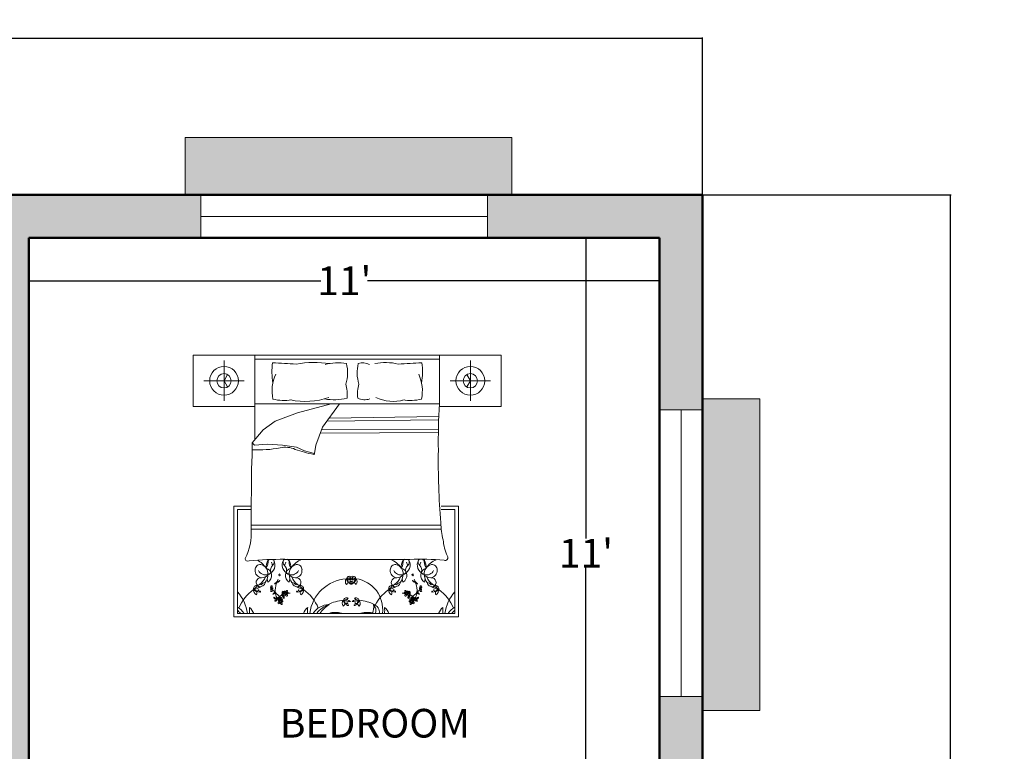
# Model space of a CAD drawing. Units: inches. Extents: x -28 to 544, y -640 to 52.
# Tile 11 of 11: x 338 to 544, y -109 to 44. Entities that reach past the tile are written whole.
import ezdxf

# ---------------------------------------------------------------- set-up
doc = ezdxf.new("R2010")
doc.units = ezdxf.units.IN
doc.header["$MEASUREMENT"] = 0
for name, color, linetype, lineweight in [('A-ANNO-DIMS', 2, 'Continuous', 18), ('A-AREA-IDEN', 7, 'Continuous', 25), ('A-FURN', 8, 'Continuous', 18), ('A-GLAZ', 4, 'Continuous', 20), ('A-ROOF', 8, 'Continuous', 18), ('A-ROOF-PATT', 252, 'Continuous', 13), ('A-WALL', 7, 'Continuous', 50), ('A-WALL-PATT', 5, 'Continuous', 13)]:
    doc.layers.add(name, color=color, linetype=linetype, lineweight=lineweight)
doc.styles.get("Standard").update_dxf_attribs({"font": 'arial.ttf'})
doc.dimstyles.get("Standard").update_dxf_attribs({"dimtxt": 0.18, "dimasz": 0.18, "dimexe": 0.18, "dimexo": 0.0625, "dimgap": 0.09, "dimtad": 0, "dimtih": 1, "dimtoh": 1, "dimdec": 0, "dimzin": 0, "dimdsep": 46, "dimlunit": 3, "dimtxsty": 'Standard', "dimcen": 0.09, "dimadec": 0, "dimazin": 0, "dimtfac": 1, "dimtdec": 0, "dimtofl": 0, "dimtmove": 0, "dimatfit": 3, "dimfxl": 1, "dimtolj": 1, "dimtzin": 0, "dimarcsym": 0})

# ---------------------------------------------------------------- blocks, each defined once
blk = doc.blocks.new('*D7')
at = {"layer": 'A-ANNO-DIMS', "color": 0, "lineweight": -2, "transparency": 16777216}
for p, q in [((456.03, -1.42), (456.03, -64.14)), ((456.09, -1.24), (456.21, -1.24)), ((456.03, -133.06), (456.03, -70.34)), ((456.09, -133.24), (456.21, -133.24))]:
    blk.add_line(p, q, dxfattribs=at)
at = {"layer": 'A-ANNO-DIMS', "color": 0, "transparency": 16777216}
for points in [[(456, -1.42), (456.06, -1.42), (456.03, -1.24)], [(456, -133.06), (456.06, -133.06), (456.03, -133.24)]]:
    blk.add_solid(points, dxfattribs=at)
at = {"layer": 'Defpoints', "color": 0, "transparency": 16777216}
for p in [(456.03, -1.24), (456.03, -133.24), (456.03, -133.24)]:
    blk.add_point(p, dxfattribs=at)
at = {"layer": 'A-ANNO-DIMS', "color": 0, "transparency": 16777216, "insert": (456.03, -67.24), "char_height": 6, "attachment_point": 5}
blk.add_mtext("\\A1;11'", dxfattribs=at)
blk = doc.blocks.new('*D8')
at = {"layer": 'A-ANNO-DIMS', "color": 0, "lineweight": -2, "transparency": 16777216}
for p, q in [((339.44, -16.04), (339.44, -10.04)), ((339.62, -10.22), (400.55, -10.22)), ((471.26, -10.22), (410.34, -10.22)), ((471.44, -16.04), (471.44, -10.04))]:
    blk.add_line(p, q, dxfattribs=at)
at = {"layer": 'A-ANNO-DIMS', "color": 0, "transparency": 16777216}
for points in [[(339.62, -10.19), (339.62, -10.25), (339.44, -10.22)], [(471.26, -10.19), (471.26, -10.25), (471.44, -10.22)]]:
    blk.add_solid(points, dxfattribs=at)
at = {"layer": 'Defpoints', "color": 0, "transparency": 16777216}
for p in [(471.44, -10.22), (339.44, -16.1), (471.44, -16.1)]:
    blk.add_point(p, dxfattribs=at)
at = {"layer": 'A-ANNO-DIMS', "color": 0, "transparency": 16777216, "insert": (405.44, -10.22), "char_height": 6, "attachment_point": 5}
blk.add_mtext("\\A1;11'", dxfattribs=at)
blk = doc.blocks.new('*D27')
at = {"layer": 'A-ANNO-DIMS', "color": 0, "lineweight": -2, "transparency": 16777216}
for p, q in [((16.94, 7.82), (16.94, 40.69)), ((17.12, 40.51), (238.3, 40.51)), ((480.26, 40.51), (259.09, 40.51)), ((480.44, 7.82), (480.44, 40.69))]:
    blk.add_line(p, q, dxfattribs=at)
at = {"layer": 'A-ANNO-DIMS', "color": 0, "transparency": 16777216}
for points in [[(17.12, 40.54), (17.12, 40.48), (16.94, 40.51)], [(480.26, 40.54), (480.26, 40.48), (480.44, 40.51)]]:
    blk.add_solid(points, dxfattribs=at)
at = {"layer": 'Defpoints', "color": 0, "transparency": 16777216}
for p in [(480.44, 40.51), (16.94, 7.76), (480.44, 7.76)]:
    blk.add_point(p, dxfattribs=at)
at = {"layer": 'A-ANNO-DIMS', "color": 0, "transparency": 16777216, "insert": (248.69, 40.51), "char_height": 6, "attachment_point": 5}
blk.add_mtext('\\A1;38\'-8"', dxfattribs=at)
blk = doc.blocks.new('*D28')
at = {"layer": 'A-ANNO-DIMS', "color": 0, "lineweight": -2, "transparency": 16777216}
for p, q in [((480.51, 7.76), (532.47, 7.76)), ((532.29, 7.58), (532.29, -286.84)), ((532.29, -587.56), (532.29, -293.14)), ((480.51, -587.74), (532.47, -587.74))]:
    blk.add_line(p, q, dxfattribs=at)
at = {"layer": 'A-ANNO-DIMS', "color": 0, "transparency": 16777216}
for points in [[(532.26, 7.58), (532.32, 7.58), (532.29, 7.76)], [(532.26, -587.56), (532.32, -587.56), (532.29, -587.74)]]:
    blk.add_solid(points, dxfattribs=at)
at = {"layer": 'Defpoints', "color": 0, "transparency": 16777216}
for p in [(480.44, 7.76), (480.44, -587.74), (532.29, -587.74)]:
    blk.add_point(p, dxfattribs=at)
at = {"layer": 'A-ANNO-DIMS', "color": 0, "transparency": 16777216, "insert": (532.29, -289.99), "char_height": 6, "attachment_point": 5}
blk.add_mtext('\\A1;49\'-8"', dxfattribs=at)
blk = doc.blocks.new('BED-DOUBLE-HEADBOARD-64')
for p, q in [((0, 54.82), (64.46, 54.82)), ((6.45, 45.23), (6.45, 53.66)), ((12.89, 54.82), (12.89, 37.12)), ((51.57, 53.99), (12.89, 53.99)), ((58.01, 45.23), (58.01, 53.66)), ((10.66, 49.44), (2.23, 49.44)), ((53.8, 49.44), (62.22, 49.44)), ((12.89, 44.63), (51.57, 44.63)), ((21.84, 42.71), (28.87, 44.63)), ((30.6, 44.63), (27.07, 39.71)), ((17.14, 41.02), (21.84, 42.71)), ((51.37, 41.29), (27.96, 40.96)), ((51.39, 41.95), (28.44, 41.63)), ((12.31, 36.45), (14.66, 39.19)), ((14.66, 39.19), (17.14, 41.02)), ((27.07, 39.71), (25.63, 35.93)), ((51.33, 39.26), (26.86, 39.16)), ((51.34, 38.6), (26.61, 38.5)), ((12.84, 35.93), (12.31, 36.45)), ((15.45, 36.19), (12.84, 35.93)), ((18.71, 35.93), (15.45, 36.19)), ((21.58, 35.54), (18.71, 35.93)), ((23.28, 34.76), (21.58, 35.54)), ((25.63, 35.93), (25.37, 34.23)), ((25.37, 34.23), (23.28, 34.76)), ((8.51, 23.22), (12.15, 23.22)), ((8.51, 0), (8.51, 23.22)), ((51.92, 23.22), (55.5, 23.22)), ((55.5, 23.22), (55.5, 0)), ((12.15, 22.47), (9.25, 22.47)), ((9.25, 22.47), (9.25, 0.75)), ((54.75, 22.47), (51.91, 22.47)), ((54.75, 0.75), (54.75, 22.47)), ((51.86, 19.2), (12.15, 19.2)), ((51.92, 18.4), (12.15, 18.4)), ((45.31, 12.06), (19.14, 12.06)), ((15.61, 7.28), (15.46, 8.01)), ((20.11, 7.28), (20.25, 8.01)), ((43.9, 7.28), (43.75, 8.01)), ((48.4, 7.28), (48.54, 8.01)), ((55.5, 0), (8.51, 0)), ((9.25, 0.75), (54.75, 0.75))]:
    blk.add_line(p, q)
for points in [[(12.89, 44.07), (0, 44.07), (0, 54.82)], [(51.57, 54.82), (51.57, 44.07), (64.46, 44.07), (64.46, 54.82)], [(6.45, 49.44), (7.2, 50.75)], [(58.01, 49.44), (57.26, 50.75)], [(6.45, 49.44), (7.2, 48.14)], [(58.01, 49.44), (57.26, 48.14)]]:
    blk.add_lwpolyline(points)
for points in [[(16.59, 53.21, 0.074897), (16.67, 49, -0.472817)], [(31.93, 48.76, 0.14099), (32.06, 53.06, 0.235245)], [(34.68, 48.76, -0.14099), (34.55, 53.06, -0.235245)], [(47.86, 53.21, -0.074897), (47.78, 49, 0.472817)], [(12.18, 30.55, 0.001242), (12.15, 18.32, -0.127202), (10.86, 12.22)], [(51.84, 19.71, 0.056112), (52.31, 16.16, 0.095341), (53.21, 12.74)]]:
    blk.add_lwpolyline(points, format="xyb")
for centre, radius in [((6.45, 49.44), 3.01), ((58.01, 49.44), 3.01), ((6.45, 49.44), 1.5), ((58.01, 49.44), 1.5), ((19.33, 4.95), 0.164), ((44.68, 4.95), 0.164), ((18.26, 3.22), 0.164), ((45.75, 3.22), 0.164)]:
    blk.add_circle(centre, radius)
for centre, radius, start, end in [((52.12, 666.62), 614.44, 266.68521, 267.14978), ((25.43, 29.89), 23.38, 82.2196, 99.497), ((30.36, 41.7), 11.49, 81.5249, 103.96), ((35.43, 50), 3.19, 63.3437, 106.1026), ((40.21, 41.93), 11.33, 76.3427, 101.1841), ((12.34, 666.62), 614.44, 272.85022, 273.31479), ((24.81, 47.31), 8.31, 155.1316, 191.7583), ((39.65, 47.31), 8.31, 348.2417, 24.8684), ((24.33, 46.61), 7.9, 354.0129, 15.8293), ((42.28, 46.61), 7.9, 164.1707, 185.9871), ((18.89, 53.96), 8.64, 255.1039, 281.0369), ((23.44, 60.1), 14.98, 258.0397, 289.2615), ((29.51, 56.83), 11.37, 259.8617, 283.6238), ((35.87, 48.88), 3.42, 245.0183, 288.5407), ((41.84, 53.33), 8.2, 243.8761, 286.1746), ((45.56, 53.96), 8.64, 258.9631, 284.8961), ((167.11, 36.75), 115.82, 176.1, 180.9282), ((-46.79, 34.85), 59.12, 355.8294, 1.553), ((13.42, 59.28), 24.33, 267.4519, 281.3392), ((19.23, 30.28), 5.25, 66.2616, 101.3392), ((29.84, 58.59), 25, 250.1194, 259.3383), ((25.22, 34.18), 0.156, 268.8623, 19.7536), ((202.37, 32.54), 151.08, 179.1145, 184.8735), ((52.73, 12.42), 0.588, 246.5219, 33.8264), ((11.45, 12.27), 0.595, 183.98, 297.3412), ((18.37, -55.03), 67.1, 89.3433, 95.6887), ((14.04, 9.87), 1.09, 84.4856, 181.0538), ((11.2, 7.52), 4.88, 33.6671, 63.2997), ((13.71, 9.06), 1.94, 355.2933, 76.921), ((17.74, 10.43), 2.49, 145.785, 184.7304), ((12.99, 11.59), 2.67, 328.8218, 9.1554), ((16.3, 11.35), 0.776, 120.0293, 142.325), ((15.06, 10.89), 2.05, 289.2822, 29.1751), ((17.48, 9.79), 1.32, 131.5653, 195.1471), ((14.75, 10.52), 1.85, 7.436, 29.9149), ((15.97, 11.5), 0.964, 311.5653, 23.8354), ((16.3, 11.35), 0.776, 44.4517, 63.558), ((20.66, 10.89), 2.05, 150.8249, 250.7178), ((19.75, 11.5), 0.964, 156.1646, 228.4347), ((19.42, 11.35), 0.776, 113.229, 135.5483), ((18.23, 9.79), 1.32, 344.8529, 48.4347), ((20.97, 10.52), 1.85, 150.0851, 172.564), ((19.42, 11.35), 0.776, 37.675, 66.7144), ((17.98, 10.43), 2.49, 355.2696, 34.215), ((22.73, 11.59), 2.67, 169.7133, 211.1782), ((22.01, 9.06), 1.94, 103.079, 184.7067), ((24.52, 7.52), 4.88, 111.4941, 146.3329), ((21.68, 9.87), 1.09, 358.9462, 95.5144), ((42.33, 9.87), 1.09, 84.4856, 181.0538), ((39.49, 7.52), 4.88, 33.6671, 68.5059), ((42, 9.06), 1.94, 355.2933, 76.921), ((46.03, 10.43), 2.49, 145.785, 184.7304), ((41.28, 11.59), 2.67, 328.8218, 10.2867), ((44.58, 11.35), 0.776, 113.2856, 142.325), ((43.35, 10.89), 2.05, 289.2822, 29.1751), ((45.77, 9.79), 1.32, 131.5653, 195.1471), ((43.04, 10.52), 1.85, 7.436, 29.9149), ((44.58, 11.35), 0.776, 44.4517, 66.7144), ((44.26, 11.5), 0.964, 311.5653, 23.8354), ((47.29, -50.63), 62.72, 85.2402, 91.8035), ((48.95, 10.89), 2.05, 150.8249, 250.7178), ((48.04, 11.5), 0.964, 156.1646, 228.4347), ((47.71, 11.35), 0.776, 106.6343, 135.5483), ((46.52, 9.79), 1.32, 344.8529, 48.4347), ((49.26, 10.52), 1.85, 150.0851, 172.564), ((47.71, 11.35), 0.776, 37.675, 72.5814), ((46.27, 10.43), 2.49, 355.2696, 34.215), ((51.02, 11.59), 2.67, 169.249, 211.1782), ((50.3, 9.06), 1.94, 103.079, 184.7067), ((52.81, 7.52), 4.88, 113.6453, 146.3329), ((49.97, 9.87), 1.09, 358.9462, 95.5144), ((14.49, 9.71), 1.54, 174.9449, 262.8857), ((15.09, 10.3), 1.5, 201.5819, 291.4221), ((12.21, 9.36), 3.04, 301.2614, 341.7045), ((14.22, 10.05), 1.87, 272.3591, 324.0401), ((12.19, 9.11), 3.46, 326.2883, 356.5076), ((14.81, 8.67), 1.6, 299.9085, 73.1337), ((17.74, 10.43), 2.49, 212.7011, 216.3445), ((15.82, 9.34), 0.4, 257.3041, 15.1471), ((18.04, 8.74), 0.124, 102.7051, 280.4384), ((18.03, 8.81), 0.202, 280.4384, 100.4136), ((20.91, 8.67), 1.6, 106.8663, 240.0915), ((19.9, 9.34), 0.4, 164.8529, 282.6959), ((17.98, 10.43), 2.49, 323.6555, 327.2989), ((21.5, 10.05), 1.87, 215.9599, 267.6409), ((20.63, 10.3), 1.5, 248.5779, 338.4181), ((23.53, 9.11), 3.46, 183.4924, 213.7117), ((23.5, 9.36), 3.04, 198.2955, 238.7386), ((21.23, 9.71), 1.54, 277.1143, 5.0551), ((32.74, 7.81), 0.698, 63.0274, 163.8037), ((32.04, 9.44), 1.44, 271.4585, 315.3727), ((33.41, 7.81), 0.698, 16.1963, 116.9726), ((34.12, 9.44), 1.44, 224.6273, 268.5415), ((42.78, 9.71), 1.54, 174.9449, 262.8857), ((43.38, 10.3), 1.5, 201.5819, 291.4221), ((40.5, 9.36), 3.04, 301.2614, 341.7045), ((42.51, 10.05), 1.87, 272.3591, 324.0401), ((40.47, 9.11), 3.46, 326.2883, 356.5076), ((43.1, 8.67), 1.6, 299.9085, 73.1337), ((46.03, 10.43), 2.49, 212.7011, 216.3445), ((44.11, 9.34), 0.4, 257.3041, 15.1471), ((45.98, 8.81), 0.202, 79.5864, 259.5616), ((45.96, 8.74), 0.124, 259.5616, 77.2949), ((49.2, 8.67), 1.6, 106.8663, 240.0915), ((48.18, 9.34), 0.4, 164.8529, 282.6959), ((46.27, 10.43), 2.49, 323.6555, 327.2989), ((49.79, 10.05), 1.87, 215.9599, 267.6409), ((48.91, 10.3), 1.5, 248.5779, 338.4181), ((51.82, 9.11), 3.46, 183.4924, 213.7117), ((51.79, 9.36), 3.04, 198.2955, 238.7386), ((49.52, 9.71), 1.54, 277.1143, 5.0551), ((13.31, 5.89), 0.698, 92.9516, 193.728), ((11.89, 6.95), 1.44, 301.3827, 345.2969), ((13.71, 4.95), 1.33, 75.4653, 144.2343), ((11.36, 11.48), 5.89, 282.5173, 297.1824), ((14.13, 7.23), 0.967, 80.264, 250.8688), ((13.93, 6.18), 0.593, 63.9755, 143.2681), ((13.9, 7.52), 1.21, 265.969, 344.3045), ((15.2, 5.91), 1.29, 96.1662, 141.5825), ((16.38, 6.18), 0.274, 101.5637, 142.6358), ((16.34, 6.08), 0.157, 91.1081, 181.8675), ((16.16, 6.39), 0.395, 288.7263, 352.5032), ((16.42, 6.37), 0.127, 345.2356, 144.9248), ((17.33, 6.82), 0.338, 101.3256, 154.4621), ((16.85, 7.97), 1.02, 280.2588, 300.656), ((17.08, 8.78), 1.82, 268.3264, 277.1302), ((22.51, 5.49), 5.34, 163.5842, 183.8277), ((16.63, 7.96), 1.04, 308.2101, 316.3071), ((17.26, 7.28), 0.309, 278.3432, 4.2869), ((17.09, 7.55), 0.54, 300.656, 332.6341), ((17.5, 7.2), 0.131, 55.7657, 157.4417), ((22.51, 5.49), 5.34, 153.0032, 159.8941), ((17.7, 7.32), 0.131, 84.3784, 186.0543), ((17.58, 7.85), 0.54, 269.1859, 301.164), ((17.74, 7.57), 0.309, 237.5332, 323.4768), ((17.44, 8.45), 1.04, 285.5129, 293.6099), ((18.11, 7.28), 0.338, 87.3579, 140.4944), ((17.33, 8.26), 1.02, 301.164, 321.5612), ((16.5, 8.43), 1.82, 324.6898, 333.4936), ((20.52, 5.91), 1.29, 38.4175, 83.8338), ((21.82, 7.52), 1.21, 195.6955, 274.031), ((21.59, 7.23), 0.967, 289.1312, 99.736), ((21.78, 6.18), 0.593, 36.7319, 116.0245), ((22, 4.95), 1.33, 35.7657, 104.5347), ((24.36, 11.48), 5.89, 242.8176, 257.4827), ((22.41, 5.89), 0.698, 346.272, 87.0484), ((23.83, 6.95), 1.44, 194.7031, 238.6173), ((32.73, -0.39), 8.42, 94.4623, 172.255), ((32.77, 7.38), 0.933, 137.7873, 219.1145), ((31.71, 7.41), 0.703, 298.5391, 58.3627), ((32.62, 6.79), 1.33, 45.5411, 114.3101), ((33.84, 13.62), 5.89, 252.593, 267.2582), ((32.76, 7.98), 0.689, 177.7585, 283.852), ((34.09, 8.69), 2.13, 198.9159, 238.011), ((33.53, 6.79), 1.33, 65.6899, 134.4589), ((32.32, 13.62), 5.89, 272.7418, 287.407), ((32.91, 7.4), 0.0911, 283.852, 219.9245), ((33.02, 6.98), 0.105, 238.011, 71.5592), ((33.03, 7.03), 0.0508, 71.5592, 188.0167), ((33.14, 6.98), 0.105, 108.4408, 301.989), ((33.12, 7.03), 0.0508, 351.9833, 108.4408), ((32.07, 8.69), 2.13, 301.989, 341.0841), ((33.24, 7.43), 0.0549, 320.1909, 256.0209), ((33.39, 7.98), 0.689, 256.148, 2.2415), ((34.45, 7.41), 0.703, 121.6373, 241.4609), ((33.39, 7.38), 0.933, 320.8855, 42.2127), ((33.15, 1.56), 6.51, 352.8636, 81.8197), ((41.6, 5.89), 0.698, 92.9516, 193.728), ((40.18, 6.95), 1.44, 301.3827, 345.2969), ((42, 4.95), 1.33, 75.4653, 144.2343), ((39.65, 11.48), 5.89, 282.5173, 297.1824), ((42.42, 7.23), 0.967, 80.264, 250.8688), ((42.22, 6.18), 0.593, 63.9755, 143.2681), ((42.19, 7.52), 1.21, 265.969, 344.3045), ((43.49, 5.91), 1.29, 96.1662, 141.5825), ((46.68, 8.26), 1.02, 218.4388, 238.836), ((45.9, 7.28), 0.338, 39.5056, 92.6421), ((47.51, 8.43), 1.82, 206.5064, 215.3102), ((46.27, 7.57), 0.309, 216.5232, 302.4668), ((46.43, 7.85), 0.54, 238.836, 270.8141), ((46.57, 8.45), 1.04, 246.3901, 254.4871), ((41.5, 5.49), 5.34, 20.1059, 26.9968), ((46.31, 7.32), 0.131, 353.9457, 95.6216), ((46.51, 7.2), 0.131, 22.5583, 124.2343), ((46.75, 7.28), 0.309, 175.7131, 261.6568), ((46.92, 7.55), 0.54, 207.3659, 239.344), ((41.5, 5.49), 5.34, 356.1723, 16.4158), ((47.38, 7.96), 1.04, 223.6929, 231.7899), ((47.16, 7.97), 1.02, 239.344, 259.7412), ((46.93, 8.78), 1.82, 262.8698, 271.6736), ((46.67, 6.82), 0.338, 25.5379, 78.6744), ((47.58, 6.37), 0.127, 35.0752, 194.7644), ((47.85, 6.39), 0.395, 187.4968, 251.2737), ((47.67, 6.08), 0.157, 358.1325, 88.8919), ((47.63, 6.18), 0.274, 37.3642, 78.4363), ((50.11, 7.52), 1.21, 195.6955, 274.031), ((48.81, 5.91), 1.29, 38.4175, 83.8338), ((49.87, 7.23), 0.967, 289.1312, 99.736), ((50.07, 6.18), 0.593, 36.7319, 116.0245), ((50.29, 4.95), 1.33, 35.7657, 104.5347), ((52.65, 11.48), 5.89, 242.8176, 257.4827), ((52.12, 6.95), 1.44, 194.7031, 238.6173), ((50.69, 5.89), 0.698, 346.272, 87.0484), ((2.99, -0.39), 8.42, 7.745, 41.8856), ((17.39, -1.22), 8.42, 124.3865, 158.5908), ((13.55, 5.53), 0.933, 167.7115, 249.0387), ((12.61, 5.02), 0.703, 328.4633, 88.2869), ((14.04, 7.33), 2.13, 228.8402, 267.9352), ((13.24, 6.05), 0.689, 207.6827, 313.7762), ((13.66, 5.62), 0.0911, 313.7762, 249.7183), ((13.95, 5.36), 0.0508, 101.4834, 217.9409), ((13.96, 5.31), 0.105, 267.9352, 101.4834), ((16.15, 5.92), 0.164, 273.2768, 86.7232), ((16.37, 5.62), 0.271, 217.7621, 259.0403), ((16.66, 5.98), 0.498, 203.4276, 227.6104), ((16.51, 5.76), 0.339, 80.3487, 133.6538), ((16.45, 6.04), 0.269, 229.7889, 317.6792), ((16.14, 5.47), 0.381, 355.053, 68.3618), ((16.44, 5.41), 0.537, 83.0852, 105.7171), ((16.4, 5.45), 0.126, 232.4737, 355.053), ((12.72, 0.95), 6.12, 43.1541, 52.0459), ((16.54, 5.96), 0.141, 317.6792, 80.3487), ((16.95, 4.65), 0.338, 101.3256, 154.4621), ((16.46, 5.8), 1.02, 280.2588, 300.656), ((16.7, 6.61), 1.82, 268.3264, 277.1302), ((16.24, 5.79), 1.04, 308.2101, 316.3071), ((17.06, 4.06), 0.183, 146.8636, 236.9021), ((19.65, 8.09), 4.8, 235.1882, 238.8844), ((17.38, 4.32), 0.496, 199.4799, 267.6828), ((16.88, 5.11), 0.309, 278.3432, 4.2869), ((16.71, 5.39), 0.54, 300.656, 332.6341), ((17.11, 5.03), 0.131, 55.7657, 157.4417), ((19.85, 5.36), 2.68, 184.756, 209.2041), ((23.71, 11.06), 8.81, 222.2412, 232.1744), ((20.13, 1.8), 3.21, 120.544, 139.818), ((18.07, 5.19), 0.748, 304.5369, 16.3699), ((18.47, 5.02), 0.455, 272.8499, 356.1226), ((18.15, 4.85), 0.44, 321.7607, 7.9252), ((18.24, 4.21), 0.44, 8.7227, 54.8872), ((18.27, 3.86), 0.748, 0.278, 72.111), ((19.11, 4.98), 0.529, 127.3105, 187.9252), ((18.6, 4.14), 0.455, 20.5253, 88.5375), ((19.2, 4.36), 0.529, 188.7227, 249.3375), ((18.39, 5.04), 0.544, 355.0106, 41.658), ((18.99, 4.64), 0.163, 148.0499, 225.6268), ((20.13, 1.8), 3.21, 113.0501, 113.8477), ((19.29, 4.45), 0.518, 104.7558, 148.0499), ((19, 4.82), 0.324, 247.4086, 351.4386), ((19.15, 5.17), 0.224, 126.1046, 271.4281), ((19.12, 5.24), 0.161, 353.7526, 131.7054), ((18.52, 4.1), 0.544, 334.9899, 21.6373), ((19.09, 4.81), 0.109, 262.906, 7.132), ((18.97, 5.04), 0.226, 0.0645, 61.1507), ((19.03, 5.24), 0.258, 311.8413, 355.7877), ((19.56, 5.2), 0.274, 101.5637, 176.365), ((19.55, 4.64), 0.271, 151.2196, 259.0403), ((19.52, 5.1), 0.157, 91.1081, 181.8675), ((19.85, 5), 0.498, 203.4276, 227.6104), ((19.69, 4.79), 0.339, 80.3487, 133.6538), ((19.63, 5.07), 0.269, 229.7889, 317.6792), ((19.34, 5.42), 0.395, 288.7263, 352.5032), ((19.32, 4.5), 0.381, 355.053, 68.3618), ((19.62, 4.43), 0.537, 83.0852, 105.7171), ((19.61, 5.4), 0.127, 345.2356, 144.9248), ((19.58, 4.48), 0.126, 232.4737, 355.053), ((19.72, 4.98), 0.141, 317.6792, 80.3487), ((20.13, 1.8), 3.21, 87.1071, 94.7585), ((21.75, 5.31), 0.105, 78.5166, 272.0648), ((21.68, 7.33), 2.13, 272.0648, 311.1598), ((21.77, 5.36), 0.0508, 322.0591, 78.5166), ((22.47, 6.05), 0.689, 226.2238, 332.3173), ((22.07, 5.65), 0.0549, 290.2667, 226.2271), ((23.1, 5.02), 0.703, 91.7131, 211.5367), ((22.17, 5.53), 0.933, 290.9613, 12.2885), ((18.33, -1.22), 8.42, 21.4092, 55.6135), ((45.68, -1.22), 8.42, 124.3865, 158.5908), ((41.84, 5.53), 0.933, 167.7115, 249.0387), ((41.53, 6.05), 0.689, 207.6827, 313.7762), ((42.33, 7.33), 2.13, 228.8402, 267.9352), ((40.9, 5.02), 0.703, 328.4633, 88.2869), ((41.95, 5.62), 0.0911, 313.7762, 249.7183), ((42.24, 5.36), 0.0508, 101.4834, 217.9409), ((42.25, 5.31), 0.105, 267.9352, 101.4834), ((43.88, 1.8), 3.21, 85.2415, 92.8929), ((44.29, 4.98), 0.141, 99.6513, 222.3208), ((44.38, 5.07), 0.269, 222.3208, 310.2111), ((44.32, 4.79), 0.339, 46.3462, 99.6513), ((44.4, 5.4), 0.127, 35.0752, 194.7644), ((44.67, 5.42), 0.395, 187.4968, 251.2737), ((44.68, 4.5), 0.381, 111.6382, 184.947), ((44.43, 4.48), 0.126, 184.947, 307.5263), ((44.38, 4.43), 0.537, 74.2829, 96.9148), ((44.49, 5.1), 0.157, 358.1325, 88.8919), ((44.45, 5.2), 0.274, 3.635, 78.4363), ((44.16, 5), 0.498, 312.3896, 336.5724), ((44.45, 4.64), 0.271, 280.9597, 28.7804), ((45.01, 4.82), 0.324, 188.5614, 292.5914), ((44.88, 5.24), 0.161, 48.2946, 186.2474), ((44.98, 5.24), 0.258, 184.2123, 228.1587), ((45.03, 5.04), 0.226, 118.8493, 179.9355), ((44.92, 4.81), 0.109, 172.868, 277.094), ((44.86, 5.17), 0.224, 268.5719, 53.8954), ((44.72, 4.45), 0.518, 31.9501, 75.2442), ((45.48, 4.1), 0.544, 158.3627, 205.0101), ((45.4, 4.14), 0.455, 91.4625, 159.4747), ((45.74, 3.86), 0.748, 107.889, 179.722), ((44.8, 4.36), 0.529, 290.6625, 351.2773), ((45.62, 5.04), 0.544, 138.342, 184.9894), ((45.53, 5.02), 0.455, 183.8774, 267.1501), ((43.88, 1.8), 3.21, 66.1523, 66.9499), ((45.02, 4.64), 0.163, 314.3732, 31.9501), ((45.93, 5.19), 0.748, 163.6301, 235.4631), ((44.89, 4.98), 0.529, 352.0748, 52.6895), ((45.76, 4.21), 0.44, 125.1128, 171.2773), ((45.85, 4.85), 0.44, 172.0748, 218.2393), ((43.88, 1.8), 3.21, 40.182, 59.456), ((40.3, 11.06), 8.81, 307.8256, 317.7588), ((44.15, 5.36), 2.68, 330.7959, 355.244), ((46.63, 4.32), 0.496, 272.3172, 340.5201), ((51.29, 0.95), 6.12, 127.9541, 136.8459), ((46.9, 5.03), 0.131, 22.5583, 124.2343), ((47.13, 5.11), 0.309, 175.7131, 261.6568), ((47.3, 5.39), 0.54, 207.3659, 239.344), ((44.36, 8.09), 4.8, 301.1156, 304.8118), ((47.77, 5.79), 1.04, 223.6929, 231.7899), ((47.55, 5.8), 1.02, 239.344, 259.7412), ((46.94, 4.06), 0.183, 303.0979, 33.1364), ((47.31, 6.61), 1.82, 262.8698, 271.6736), ((47.06, 4.65), 0.338, 25.5379, 78.6744), ((47.47, 5.96), 0.141, 99.6513, 222.3208), ((47.56, 6.04), 0.269, 222.3208, 310.2111), ((47.5, 5.76), 0.339, 46.3462, 99.6513), ((47.86, 5.47), 0.381, 111.6382, 184.947), ((47.61, 5.45), 0.126, 184.947, 307.5263), ((47.57, 5.41), 0.537, 74.2829, 96.9148), ((47.34, 5.98), 0.498, 312.3896, 336.5724), ((47.86, 5.92), 0.164, 93.2768, 266.7232), ((47.64, 5.62), 0.271, 280.9597, 322.2379), ((50.04, 5.31), 0.105, 78.5166, 272.0648), ((49.97, 7.33), 2.13, 272.0648, 311.1598), ((50.05, 5.36), 0.0508, 322.0591, 78.5166), ((50.76, 6.05), 0.689, 226.2238, 332.3173), ((50.36, 5.65), 0.0549, 290.2667, 226.2271), ((51.39, 5.02), 0.703, 91.7131, 211.5367), ((50.46, 5.53), 0.933, 290.9613, 12.2885), ((46.62, -1.22), 8.42, 21.4092, 55.6135), ((61.02, -0.39), 8.42, 138.1144, 172.255), ((17.32, 4.13), 0.427, 212.8155, 277.3992), ((17.07, 3.85), 0.496, 266.9701, 338.2913), ((14.46, 7.39), 4.8, 302.6784, 306.3746), ((17.2, 3.46), 0.183, 214.3538, 304.3923), ((17.27, 4.15), 0.19, 238.8844, 314.2646), ((17.23, 3.72), 0.427, 280.3057, 17.1958), ((17.19, 3.68), 0.19, 306.3746, 21.7548), ((17.5, 3.8), 0.143, 19.3605, 201.7548), ((17.5, 3.91), 0.143, 311.8703, 134.2646), ((20.19, 2.61), 2.86, 153.7819, 158.2913), ((17.91, 4.56), 0.748, 247.2305, 319.0635), ((17.67, 4.31), 0.44, 264.4544, 310.6188), ((19.85, 5.36), 2.68, 214.0033, 222.4917), ((17.99, 4.13), 0.455, 218.3208, 298.8162), ((17.91, 2.91), 0.163, 148.0499, 225.6268), ((18.21, 2.72), 0.518, 104.7558, 148.0499), ((17.92, 3.09), 0.324, 247.4086, 351.4386), ((18.08, 3.44), 0.224, 126.1046, 271.4281), ((18.05, 3.51), 0.161, 353.7526, 131.7054), ((18.3, 3.57), 0.529, 70.0041, 130.6188), ((18.01, 3.08), 0.109, 262.906, 7.132), ((17.9, 3.31), 0.226, 0.0645, 61.1507), ((17.95, 3.51), 0.258, 311.8413, 355.7877), ((17.96, 4.22), 0.544, 297.7043, 344.3516), ((18.48, 3.47), 0.274, 101.5637, 176.365), ((18.48, 2.91), 0.271, 151.2196, 259.0403), ((18.45, 3.37), 0.157, 91.1081, 181.8675), ((18.77, 3.27), 0.498, 203.4276, 227.6104), ((18.61, 3.06), 0.339, 80.3487, 133.6538), ((18.55, 3.34), 0.269, 229.7889, 317.6792), ((18.26, 3.68), 0.395, 288.7263, 352.5032), ((18.25, 2.77), 0.381, 355.053, 68.3618), ((18.55, 2.7), 0.537, 83.0852, 105.7171), ((18.53, 3.67), 0.127, 345.2356, 144.9248), ((18.51, 2.75), 0.126, 232.4737, 355.053), ((18.65, 3.25), 0.141, 317.6792, 80.3487), ((28.51, -1.51), 4.1, 91.272, 146.5383), ((29.98, -2.28), 5.11, 107.8504, 143.6964), ((32.67, -3.72), 7.6, 124.0123, 144.053), ((32.09, -4.9), 8.42, 94.4623, 117.4146), ((32.12, 2.87), 0.933, 137.7873, 219.1145), ((31.06, 2.9), 0.703, 298.5391, 58.3627), ((32.1, 3.3), 0.698, 63.0274, 163.8037), ((31.39, 4.93), 1.44, 271.4585, 315.3727), ((31.98, 2.28), 1.33, 45.5411, 114.3101), ((33.44, 4.19), 2.13, 198.9159, 238.011), ((33.19, 9.11), 5.89, 252.593, 267.2582), ((32.12, 3.47), 0.689, 177.7585, 283.852), ((32.26, 2.89), 0.0911, 283.852, 219.9245), ((32.37, 2.47), 0.105, 238.011, 71.5592), ((32.39, 2.52), 0.0508, 71.5592, 188.0167), ((34.18, 2.28), 1.33, 65.6899, 134.4589), ((32.96, 9.11), 5.89, 272.7418, 287.407), ((33.78, 2.47), 0.105, 108.4408, 301.989), ((34.06, 3.3), 0.698, 16.1963, 116.9726), ((34.76, 4.93), 1.44, 224.6273, 268.5415), ((33.77, 2.52), 0.0508, 351.9833, 108.4408), ((33.89, 2.92), 0.0549, 320.1909, 256.0209), ((32.71, 4.19), 2.13, 301.989, 341.0841), ((34.04, 3.47), 0.689, 256.148, 2.2415), ((35.09, 2.9), 0.703, 121.6373, 241.4609), ((34.03, 2.87), 0.933, 320.8855, 42.2127), ((34.07, -4.9), 8.42, 62.5854, 85.5377), ((34, 2.15), 3.77, 338.117, 6.6195), ((37.45, 1.1), 1.51, 346.3898, 79.0739), ((36.32, 1.31), 1.91, 342.8609, 41.9049), ((45.36, 3.25), 0.141, 99.6513, 222.3208), ((45.45, 3.34), 0.269, 222.3208, 310.2111), ((45.39, 3.06), 0.339, 46.3462, 99.6513), ((45.47, 3.67), 0.127, 35.0752, 194.7644), ((45.74, 3.68), 0.395, 187.4968, 251.2737), ((45.76, 2.77), 0.381, 111.6382, 184.947), ((45.5, 2.75), 0.126, 184.947, 307.5263), ((45.46, 2.7), 0.537, 74.2829, 96.9148), ((45.71, 3.57), 0.529, 49.3812, 109.9959), ((46.09, 4.56), 0.748, 220.9365, 292.7695), ((46.05, 4.22), 0.544, 195.6484, 242.2957), ((45.56, 3.37), 0.157, 358.1325, 88.8919), ((45.23, 3.27), 0.498, 312.3896, 336.5724), ((45.52, 3.47), 0.274, 3.635, 78.4363), ((45.53, 2.91), 0.271, 280.9597, 28.7804), ((46.08, 3.09), 0.324, 188.5614, 292.5914), ((46.02, 4.13), 0.455, 241.1838, 321.6792), ((45.96, 3.51), 0.161, 48.2946, 186.2474), ((46.05, 3.51), 0.258, 184.2123, 228.1587), ((46.11, 3.31), 0.226, 118.8493, 179.9355), ((45.99, 3.08), 0.109, 172.868, 277.094), ((45.93, 3.44), 0.224, 268.5719, 53.8954), ((45.79, 2.72), 0.518, 31.9501, 75.2442), ((46.34, 4.31), 0.44, 229.3812, 275.5456), ((44.15, 5.36), 2.68, 317.5083, 325.9967), ((46.1, 2.91), 0.163, 314.3732, 31.9501), ((46.78, 3.72), 0.427, 162.8042, 259.6943), ((46.51, 3.91), 0.143, 45.7354, 228.1297), ((46.51, 3.8), 0.143, 338.2452, 160.6395), ((43.82, 2.61), 2.86, 21.7087, 26.2181), ((46.93, 3.85), 0.496, 201.7087, 273.0299), ((46.74, 4.15), 0.19, 225.7354, 301.1156), ((46.69, 4.13), 0.427, 262.6008, 327.1845), ((46.82, 3.68), 0.19, 158.2452, 233.6254), ((49.55, 7.39), 4.8, 233.6254, 237.3216), ((46.81, 3.46), 0.183, 235.6077, 325.6462), ((7.21, -1.51), 4.1, 33.4617, 60.1116), ((5.74, -2.28), 5.11, 36.3036, 46.4814), ((9.51, -0.57), 3.42, 22.5547, 48.9546), ((0.13, 1.27), 11.65, 357.4081, 3.6519), ((26.21, -0.57), 3.42, 131.0454, 157.4453), ((35.58, 1.27), 11.65, 176.3481, 182.5919), ((29.73, -3.68), 4.63, 73.5431, 107.0202), ((31.56, -6.06), 6.84, 94.3787, 95.6357), ((35.17, -10.75), 12.23, 109.7217, 109.9028), ((36.42, -3.68), 4.63, 72.9798, 106.4569), ((34.59, -6.06), 6.84, 84.3643, 85.6213), ((30.99, -10.75), 12.23, 70.0972, 70.2783), ((28.42, 1.27), 11.65, 357.4081, 3.6519), ((37.8, -0.57), 3.42, 22.5547, 48.9546), ((54.5, -0.57), 3.42, 131.0454, 157.4453), ((63.87, 1.27), 11.65, 176.3481, 182.5919), ((56.8, -1.51), 4.1, 119.8884, 146.5383), ((58.27, -2.28), 5.11, 133.5186, 143.6964)]:
    blk.add_arc(centre, radius, start, end)
blk = doc.blocks.new('WIN-60IN')
for p, q in [((0, 9), (60, 9)), ((0, 0), (0, 9)), ((60, 9), (60, 0)), ((0, 4.5), (60, 4.5)), ((60, 0), (0, 0))]:
    blk.add_line(p, q)

msp = doc.modelspace()

# ---------------------------------------------------------------- hatches: boundary and pattern name
at = {"layer": 'A-ROOF-PATT'}
h = msp.add_hatch(color=256, dxfattribs=at)
h.dxf.hatch_style = 1
h.set_gradient(color1=(241, 235, 31), color2=(248, 153, 30))
h.paths.add_polyline_path([(124.53, 19.76), (58.75, 19.76), (58.75, 7.76), (124.53, 7.76)])
h.paths.add_polyline_path([(226.33, 19.76), (182.83, 19.76), (182.83, 7.76), (226.33, 7.76)])
h.paths.add_polyline_path([(313.67, 19.76), (271.84, 19.76), (271.84, 7.76), (313.67, 7.76)])
h.paths.add_polyline_path([(440.55, 19.76), (372.16, 19.76), (372.16, 7.76), (440.55, 7.76)])
h.paths.add_polyline_path([(492.44, -34.91), (480.44, -34.91), (480.44, -100.18), (492.44, -100.18)])
h.paths.add_polyline_path([(492.44, -151.37), (480.44, -151.37), (480.44, -179.02), (492.44, -179.02)])
h.paths.add_polyline_path([(492.44, -207.96), (480.44, -207.96), (480.44, -238.77), (492.44, -238.77)])
h.paths.add_polyline_path([(492.44, -289.99), (480.44, -289.99), (480.44, -354.53), (492.44, -354.53)])
h.paths.add_polyline_path([(492.44, -399.27), (480.44, -399.27), (480.44, -430), (492.44, -430)])
h.paths.add_polyline_path([(492.44, -475.99), (480.44, -475.99), (480.44, -546.14), (492.44, -546.14)])
h.paths.add_polyline_path([(442.7, -587.74), (368.43, -587.74), (368.43, -599.74), (442.7, -599.74)])
h.paths.add_polyline_path([(127.64, -587.74), (54.75, -587.74), (54.75, -599.74), (127.64, -599.74)])
h.paths.add_polyline_path([(16.94, -477.43), (4.94, -477.43), (4.94, -547.54), (16.94, -547.54)])
h.paths.add_polyline_path([(16.94, -399.8), (4.94, -399.8), (4.94, -430.58), (16.94, -430.58)])
h.paths.add_polyline_path([(16.94, -287.93), (4.94, -287.93), (4.94, -356.82), (16.94, -356.82)])
h.paths.add_polyline_path([(16.94, -208.93), (4.94, -208.93), (4.94, -240.18), (16.94, -240.18)])
h.paths.add_polyline_path([(16.94, -150), (4.94, -150), (4.94, -180.17), (16.94, -180.17)])
h.paths.add_polyline_path([(16.94, -32.89), (4.94, -32.89), (4.94, -101.73), (16.94, -101.73)])
at = {"layer": 'A-WALL-PATT'}
h = msp.add_hatch(color=256, dxfattribs=at)
h.dxf.hatch_style = 1
h.paths.add_polyline_path([(375.44, 7.76), (310.94, 7.76), (310.94, -1.24), (334.94, -1.24), (334.94, -133.24), (286.94, -133.24), (286.94, -137.74), (342.44, -137.74), (342.44, -133.24), (339.44, -133.24), (339.44, -1.24), (375.44, -1.24)])
h.paths.add_polyline_path([(480.44, 7.76), (435.44, 7.76), (435.44, -1.24), (471.44, -1.24), (471.44, -37.24), (480.44, -37.24)])
h.paths.add_polyline_path([(480.44, -97.24), (471.44, -97.24), (471.44, -133.24), (417.44, -133.24), (417.44, -135.49), (417.44, -137.74), (471.44, -137.74), (471.44, -152.74), (480.44, -152.74)])
h.paths.add_polyline_path([(480.44, -176.74), (471.44, -176.74), (471.44, -191.74), (387.44, -191.74), (387.44, -137.74), (389.44, -137.74), (389.44, -133.24), (370.44, -133.24), (370.44, -135.49), (370.44, -137.74), (382.94, -137.74), (382.94, -191.74), (382.94, -196.24), (382.94, -220.24), (385.19, -220.24), (387.44, -220.24), (387.44, -196.24), (471.44, -196.24), (471.44, -211.24), (480.44, -211.24)])
h.paths.add_polyline_path([(480.44, -235.24), (471.44, -235.24), (471.44, -250.24), (387.44, -250.24), (387.44, -248.24), (382.94, -248.24), (382.94, -250.24), (369.44, -250.24), (369.44, -252.49), (369.44, -254.74), (471.44, -254.74), (471.44, -290.74), (480.44, -290.74)])
h.paths.add_polyline_path([(480.44, -350.74), (471.44, -350.74), (471.44, -386.74), (339.44, -386.74), (339.44, -254.74), (341.44, -254.74), (341.44, -250.24), (334.94, -250.24), (334.94, -391.24), (471.44, -391.24), (471.44, -403.24), (480.44, -403.24)])
h.paths.add_polyline_path([(480.44, -427.24), (471.44, -427.24), (471.44, -439.24), (334.94, -439.24), (334.94, -446.74), (339.44, -446.74), (339.44, -443.74), (471.44, -443.74), (471.44, -481.24), (480.44, -481.24)])
h.paths.add_polyline_path([(480.44, -541.24), (471.44, -541.24), (471.44, -578.74), (435.44, -578.74), (435.44, -587.74), (480.44, -587.74)])
h.paths.add_polyline_path([(375.44, -578.74), (339.44, -578.74), (339.44, -474.74), (337.19, -474.74), (334.94, -474.74), (334.94, -578.74), (296.69, -578.74), (296.69, -587.74), (375.44, -587.74)])

# ---------------------------------------------------------------- linework, layer by layer
at = {"layer": 'A-ROOF'}
for p, q in [((372.16, 7.76), (372.16, 19.76)), ((372.16, 19.76), (440.55, 19.76)), ((440.55, 19.76), (440.55, 7.76)), ((480.44, -34.91), (492.44, -34.91)), ((492.44, -34.91), (492.44, -100.18)), ((492.44, -100.18), (480.44, -100.18))]:
    msp.add_line(p, q, dxfattribs=at)
at = {"layer": 'A-WALL'}
for p, q in [((16.94, 7.76), (480.44, 7.76)), ((480.44, 7.76), (480.44, -587.74)), ((339.44, -1.24), (339.44, -133.24)), ((339.44, -1.24), (471.44, -1.24)), ((471.44, -1.24), (471.44, -133.24))]:
    msp.add_line(p, q, dxfattribs=at)

# ---------------------------------------------------------------- block references
at = {"layer": 'A-FURN'}
msp.add_blockref('BED-DOUBLE-HEADBOARD-64', (373.83, -80.59), dxfattribs=at)
at = {"layer": 'A-GLAZ'}
msp.add_blockref('WIN-60IN', (375.44, -1.24), dxfattribs=at)
at = {"layer": 'A-GLAZ', "rotation": 90.00000000000003}
msp.add_blockref('WIN-60IN', (480.44, -97.24), dxfattribs=at)

# ---------------------------------------------------------------- texts
at = {"layer": 'A-AREA-IDEN', "insert": (391.95, -99.84), "char_height": 6, "attachment_point": 1}
msp.add_mtext('BEDROOM', dxfattribs=at)

# ---------------------------------------------------------------- dimensions: what is measured, and where the dimension line sits
at = {"layer": 'A-ANNO-DIMS'}
for base, p1, p2, picture, middle in [((480.44473605, 40.50985478), (16.94473605, 7.75882162), (480.44473605, 7.75882162), '*D27', (248.69473605, 40.50985478)), ((471.44, -10.22), (339.44, -16.1), (471.44, -16.1), '*D8', (405.44, -10.22))]:
    dim = msp.add_linear_dim(base=base, p1=p1, p2=p2, dimstyle='Standard', override={"dimtxt": 6, "dimclrd": 0, "dimclre": 0, "dimclrt": 0}, dxfattribs=at)
    dim.commit()
    dim.dimension.update_dxf_attribs({"geometry": picture, "text_midpoint": middle})
for base, p1, p2, picture, middle in [((532.28608123, -587.74117838), (480.44473605, 7.75882162), (480.44473605, -587.74117838), '*D28', (532.28608123, -289.99117838)), ((456.03, -133.24), (456.03, -1.24), (456.03, -133.24), '*D7', (456.03, -67.24))]:
    dim = msp.add_linear_dim(base=base, p1=p1, p2=p2, angle=90, dimstyle='Standard', override={"dimtxt": 6, "dimclrd": 0, "dimclre": 0, "dimclrt": 0}, dxfattribs=at)
    dim.commit()
    dim.dimension.update_dxf_attribs({"geometry": picture, "text_midpoint": middle})

doc.saveas('drawing.dxf')
